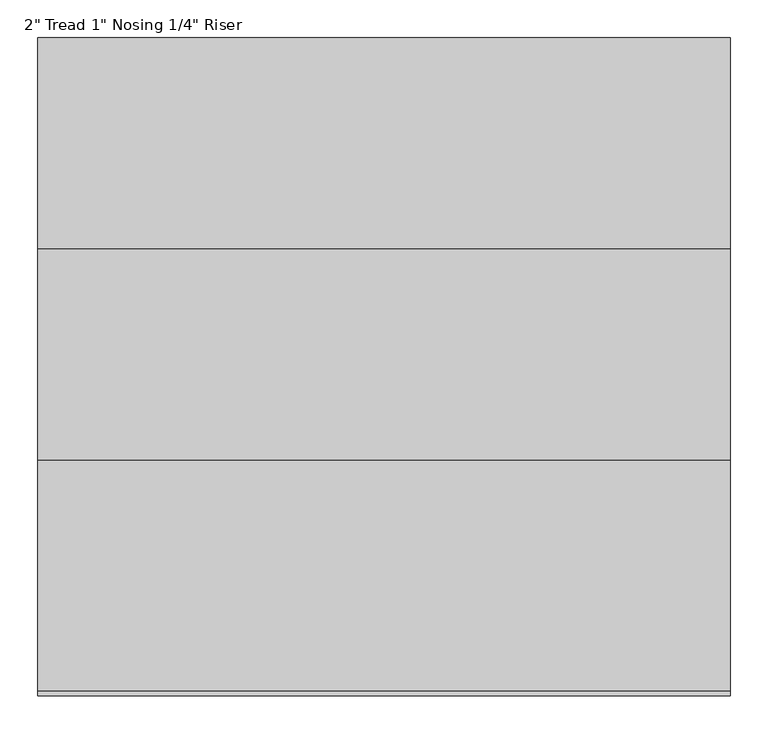
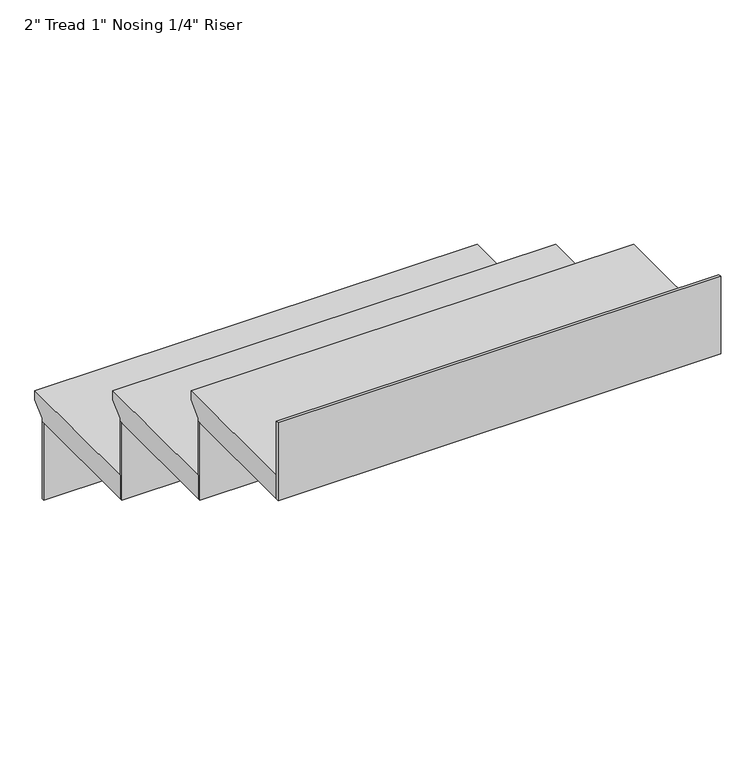
"""IFC4 building model written with IfcOpenShell, lengths in millimetres: stair flight geometry."""

from ifc_helpers import new_model, si_unit, frame, origin, place, context, project, spatial, polyline, outline, extrude, source, transform, mapped, element, save


def stair_flight_e995ea23(model_context):
    return source(origin(), model_context, "Body", "SweptSolid", [
        extrude(outline(polyline([(-19826.9851539, 52158.6172466), (-19522.1851539, 52158.6172466), (-19522.1851539, 52139.5672466), (-19547.5851539, 52114.1672466), (-19547.5851539, 52107.8172466), (-19826.9851539, 52107.8172466), (-19826.9851539, 52158.6172466)])), frame((-2296.6415084, 0.0, 0.0), z_axis=(1.0, 0.0, 0.0), x_axis=(0.0, 1.0, 0.0)), (0.0, 0.0, 1.0), 914.4),
        extrude(outline(polyline([(-2296.6415084, -19553.9351539), (-2296.6415084, -19547.5851539), (-1382.2415084, -19547.5851539), (-1382.2415084, -19553.9351539), (-2296.6415084, -19553.9351539)])), frame((0.0, 0.0, 51938.4839133), z_axis=(0.0, 0.0, 1.0), x_axis=(1.0, 0.0, 0.0)), (0.0, 0.0, 1.0), 169.3333333),
        extrude(outline(polyline([(-2296.6415084, -19833.3351539), (-2296.6415084, -19826.9851539), (-1382.2415084, -19826.9851539), (-1382.2415084, -19833.3351539), (-2296.6415084, -19833.3351539)])), frame((0.0, 0.0, 52107.8172466), z_axis=(0.0, 0.0, 1.0), x_axis=(1.0, 0.0, 0.0)), (0.0, 0.0, 1.0), 169.3333333),
        extrude(outline(polyline([(-20106.3851539, 52327.9505799), (-19801.5851539, 52327.9505799), (-19801.5851539, 52308.9005799), (-19826.9851539, 52283.5005799), (-19826.9851539, 52277.1505799), (-20106.3851539, 52277.1505799), (-20106.3851539, 52327.9505799)])), frame((-2296.6415084, 0.0, 0.0), z_axis=(1.0, 0.0, 0.0), x_axis=(0.0, 1.0, 0.0)), (0.0, 0.0, 1.0), 914.4),
        extrude(outline(polyline([(-2296.6415084, -20112.7351539), (-2296.6415084, -20106.3851539), (-1382.2415084, -20106.3851539), (-1382.2415084, -20112.7351539), (-2296.6415084, -20112.7351539)])), frame((0.0, 0.0, 52277.1505799), z_axis=(0.0, 0.0, 1.0), x_axis=(1.0, 0.0, 0.0)), (0.0, 0.0, 1.0), 169.3333333),
        extrude(outline(polyline([(-2296.6415084, -20392.1351539), (-2296.6415084, -20385.7851539), (-1382.2415084, -20385.7851539), (-1382.2415084, -20392.1351539), (-2296.6415084, -20392.1351539)])), frame((0.0, 0.0, 52446.4839133), z_axis=(0.0, 0.0, 1.0), x_axis=(1.0, 0.0, 0.0)), (0.0, 0.0, 1.0), 169.3333333),
        extrude(outline(polyline([(-20385.7851539, 52497.2839133), (-20080.9851539, 52497.2839133), (-20080.9851539, 52478.2339133), (-20106.3851539, 52452.8339133), (-20106.3851539, 52446.4839133), (-20385.7851539, 52446.4839133), (-20385.7851539, 52497.2839133)])), frame((-2296.6415084, 0.0, 0.0), z_axis=(1.0, 0.0, 0.0), x_axis=(0.0, 1.0, 0.0)), (0.0, 0.0, 1.0), 914.4),
    ])


if __name__ == "__main__":
    model = new_model("IFC4")
    model_context = context("Model", 3, world=origin())
    ifc_project = project(units=[si_unit("LENGTHUNIT", "METRE", prefix="MILLI")], contexts=[model_context])
    site = spatial("IfcSite", under=ifc_project)
    building = spatial("IfcBuilding", under=site)
    placement = place(None, origin())
    stair_flight_shape = stair_flight_e995ea23(model_context)
    element("IfcStairFlight", 1, ObjectType="2\" Tread 1\" Nosing 1/4\" Riser", at=placement, inside=building, context=model_context, shape_type="MappedRepresentation", body=[
        mapped(stair_flight_shape, transform((0.0, 0.0, 0.0), x_axis=(1.0, 0.0, 0.0), y_axis=(0.0, 1.0, 0.0), z_axis=(0.0, 0.0, 1.0))),
    ])
    save(model, "model.ifc")
